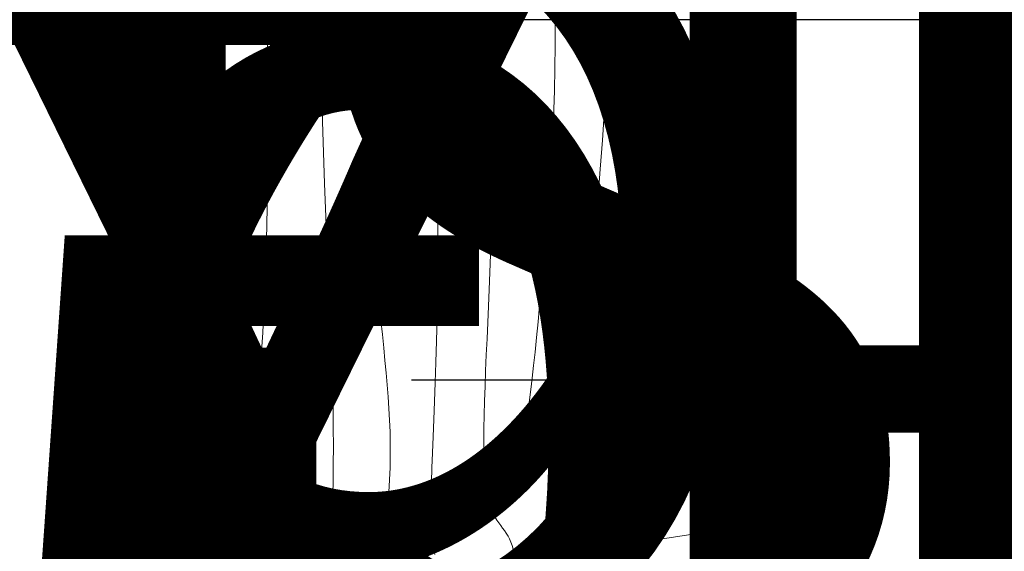
# Model space of a CAD drawing. Units: inches. Extents: x -307 to 2141, y -58 to 895.
# Tile 14 of 28: x 666 to 749, y 436 to 481. Entities that reach past the tile are written whole.
import ezdxf

# ---------------------------------------------------------------- set-up
doc = ezdxf.new("R2010")
doc.units = ezdxf.units.IN
doc.header["$MEASUREMENT"] = 0
doc.layers.add('A-ANNO-DIMS', color=2, linetype='Continuous', lineweight=18)
doc.layers.add('A-FURN', color=8, linetype='Continuous', lineweight=18)
doc.styles.get("Standard").update_dxf_attribs({"font": 'arial.ttf'})
doc.dimstyles.get("Standard").update_dxf_attribs({"dimtxt": 72, "dimasz": 48, "dimexe": 0.18, "dimexo": 0.0625, "dimgap": 0.09, "dimtad": 0, "dimtih": 1, "dimtoh": 1, "dimdec": 0, "dimrnd": 48, "dimzin": 0, "dimdsep": 46, "dimlunit": 3, "dimtxsty": 'Standard', "dimcen": 0.09, "dimadec": 0, "dimazin": 0, "dimtfac": 1, "dimtdec": 0, "dimtofl": 0, "dimtmove": 0, "dimatfit": 3, "dimfxl": 1, "dimtolj": 1, "dimtzin": 0, "dimarcsym": 0})

# ---------------------------------------------------------------- blocks, each defined once
blk = doc.blocks.new('Dining Set - 36 x 72 in.')
for p, q in [((-22, 27.5), (-6, 27.5)), ((-5.8437, 26.49966), (-6, 27.5)), ((6, 27.5), (5.8438, 26.50042)), ((6, 27.5), (22, 27.5)), ((22.1563, 26.49966), (22, 27.5)), ((-22.2304, 26), (-5.7608, 26)), ((-5.8416, 26.5), (-22.1534, 26.5)), ((-4.5152, 17.99762), (-5.7655, 25.99926)), ((5.7657, 26.00059), (4.5153, 17.99762)), ((5.7696, 26), (22.2392, 26)), ((22.1584, 26.5), (5.8466, 26.5)), ((23.4848, 17.99762), (22.2345, 25.99926)), ((36, 18), (-36, 18)), ((-36, -18), (36, -18)), ((-4.5152, -17.99762), (-5.7655, -25.99928)), ((5.7657, -26.0006), (4.5153, -17.99762)), ((23.4848, -17.99762), (22.2345, -25.99928)), ((-22.2304, -26), (-5.7608, -26)), ((-5.8416, -26.5), (-22.1534, -26.5)), ((-5.8437, -26.49967), (-6, -27.5)), ((5.7696, -26), (22.2392, -26)), ((6, -27.5), (5.8438, -26.50044)), ((22.1584, -26.5), (5.8466, -26.5)), ((22.1563, -26.49967), (22, -27.5)), ((-22, -27.5), (-6, -27.5)), ((6, -27.5), (22, -27.5))]:
    blk.add_line(p, q)
for points in [[(-22.8538, 14.81543), (-19.276, 14.6875), (-16.0362, 14.53613), (-13.0957, 14.36718), (-10.4159, 14.18652), (-7.9583, 14), (-5.6904, 13.81315), (-3.6035, 13.63021), (-1.6954, 13.45508), (0.0365, 13.29166), (1.5945, 13.14388), (2.9811, 13.01562), (4.1988, 12.9108), (5.25, 12.83333), (6.1393, 12.78613), (6.8802, 12.76823), (7.4883, 12.77767), (7.9792, 12.8125), (8.3685, 12.87077), (8.6719, 12.95052), (8.9049, 13.0498), (9.0833, 13.16666), (9.2205, 13.29899), (9.3216, 13.44401), (9.3895, 13.59879), (9.4271, 13.76041), (9.4373, 13.92594), (9.4232, 14.09245), (9.3875, 14.257), (9.3333, 14.41666), (9.2638, 14.56917), (9.1836, 14.71484), (9.0975, 14.85465), (9.0104, 14.98958), (8.9272, 15.1206), (8.8529, 15.2487), (8.7922, 15.37483), (8.75, 15.5), (8.7305, 15.62467), (8.7344, 15.74739), (8.7617, 15.86621), (8.8125, 15.97916), (8.8867, 16.08431), (8.9844, 16.17968), (9.1055, 16.26334), (9.25, 16.33333), (9.4189, 16.38802), (9.6172, 16.42708), (9.8506, 16.45052), (10.125, 16.45833), (10.4463, 16.45052), (10.8203, 16.42708), (11.2529, 16.38802), (11.75, 16.33333), (12.3184, 16.26318), (12.9694, 16.17838), (13.7151, 16.07991), (14.5677, 15.96875), (15.5395, 15.84586), (16.6426, 15.71224), (17.8893, 15.56884), (19.2917, 15.41666), (20.859, 15.25667), (22.5879, 15.08984), (24.4721, 14.91715)], [(-23.1725, 10.20442), (-18.4241, 10.19775), (-14.5677, 10.13541), (-11.4399, 10.03011), (-8.877, 9.89453), (-6.7154, 9.74137), (-4.7917, 9.58333), (-2.9698, 9.43082), (-1.2246, 9.28515), (0.4415, 9.14534), (2.026, 9.01041), (3.5266, 8.87939), (4.9408, 8.7513), (6.266, 8.62516), (7.5, 8.5), (8.6411, 8.37549), (9.6914, 8.2539), (10.6538, 8.13818), (11.5312, 8.03125), (12.3267, 7.93603), (13.043, 7.85547), (13.6831, 7.79248), (14.25, 7.75), (14.7471, 7.7303), (15.1797, 7.73307), (15.5537, 7.75732), (15.875, 7.80208), (16.1494, 7.86637), (16.3828, 7.94922), (16.5811, 8.04964), (16.75, 8.16666), (16.8944, 8.29915), (17.0143, 8.44531), (17.1089, 8.60319), (17.1771, 8.77083), (17.218, 8.94629), (17.2305, 9.1276), (17.2137, 9.31282), (17.1667, 9.5), (17.0895, 9.6875), (16.987, 9.875), (16.8649, 10.0625), (16.7292, 10.25), (16.5856, 10.4375), (16.4401, 10.625), (16.2985, 10.8125), (16.1667, 11), (16.05, 11.18733), (15.9518, 11.3737), (15.8752, 11.5581), (15.8229, 11.73958), (15.798, 11.91715), (15.8034, 12.08984), (15.842, 12.25667), (15.9167, 12.41666), (16.0295, 12.56836), (16.1784, 12.70833), (16.3605, 12.83268), (16.5729, 12.9375), (16.8127, 13.01888), (17.0768, 13.07291), (17.3625, 13.0957), (17.6667, 13.08333), (17.9894, 13.03312), (18.3418, 12.94726), (18.7382, 12.82918), (19.1927, 12.68229), (19.7195, 12.51001), (20.3327, 12.31575), (21.0465, 12.10294), (21.875, 11.875), (22.8357, 11.63354), (23.959, 11.37304), (25.2786, 11.08618)], [(-21.9946, 5.11767), (-18.4271, 5.05208), (-15.3009, 5.00602), (-12.5508, 4.97265), (-10.1112, 4.94515), (-7.9167, 4.91666), (-5.909, 4.88167), (-4.0586, 4.83984), (-2.3429, 4.79215), (-0.7396, 4.73958), (0.7739, 4.6831), (2.22, 4.6237), (3.6213, 4.56233), (5, 4.5), (6.373, 4.43782), (7.7344, 4.3776), (9.0723, 4.32129), (10.375, 4.27083), (11.6309, 4.22819), (12.8281, 4.19531), (13.9551, 4.17415), (15, 4.16666), (15.954, 4.17448), (16.819, 4.19791), (17.6001, 4.23698), (18.3021, 4.29166), (18.9299, 4.36198), (19.4883, 4.44791), (19.9823, 4.54948), (20.4167, 4.66666), (20.7969, 4.79899), (21.1302, 4.94401), (21.4245, 5.09879), (21.6875, 5.26041), (21.9271, 5.42594), (22.1511, 5.59245), (22.3672, 5.757), (22.5834, 5.91666), (22.8065, 6.06868), (23.0404, 6.21093), (23.2879, 6.34147), (23.5521, 6.45833), (23.8358, 6.55957), (24.142, 6.64323), (24.4735, 6.70735)], [(-21.6519, -0.16284), (-17.6563, 0.00521), (-14.0005, 0.12833), (-10.6523, 0.21289), (-7.5796, 0.26522), (-4.75, 0.29166), (-2.134, 0.29793), (0.2878, 0.28711), (2.5317, 0.26163), (4.6146, 0.22396), (6.5529, 0.17651), (8.3633, 0.12174), (10.0623, 0.06209), (11.6667, 0), (13.1899, -0.06201), (14.6341, -0.1211), (15.9982, -0.17432), (17.2813, -0.21875), (18.4823, -0.25147), (19.6003, -0.26953), (20.6343, -0.27002), (21.5834, -0.25), (22.4481, -0.20768), (23.2357, -0.14584), (23.9549, -0.06836), (24.6146, 0.02083)], [(-27.1843, -6.31267), (-20.084, -6.1263), (-14.469, -5.9419), (-10.1094, -5.76042), (-6.7752, -5.58285), (-4.2363, -5.41016), (-2.2629, -5.24333), (-0.625, -5.08334), (0.8708, -4.93099), (2.2715, -4.78646), (3.5872, -4.64974), (4.8281, -4.52084), (6.0046, -4.39974), (7.127, -4.28646), (8.2053, -4.18099), (9.25, -4.08334), (10.2705, -3.99382), (11.2734, -3.91407), (12.2647, -3.84603), (13.25, -3.79167), (14.2354, -3.75293), (15.2266, -3.73177), (16.2295, -3.73015), (17.25, -3.75), (18.2912, -3.79248), (19.3451, -3.85547), (20.4009, -3.93604), (21.4479, -4.03125), (22.4754, -4.13819), (23.4727, -4.25391), (24.4289, -4.37549)], [(-26.4022, -9.81299), (-18.4675, -9.62891), (-11.9839, -9.45069), (-6.7396, -9.28125), (-2.5226, -9.12354), (0.8789, -8.98047), (3.6769, -8.85498), (6.0833, -8.75), (8.2767, -8.66765), (10.3021, -8.60677), (12.1712, -8.56543), (13.8958, -8.54167), (15.4876, -8.53353), (16.9583, -8.53907), (18.3197, -8.55632), (19.5834, -8.58334), (20.7616, -8.61841), (21.8685, -8.66081), (22.9188, -8.71004), (23.9271, -8.76563), (24.9081, -8.82707)], [(-20.7312, -14.12647), (-17.0781, -14.07292), (-13.97, -14.04671), (-11.3027, -14.04297), (-8.9724, -14.05681), (-6.875, -14.08334), (-4.9224, -14.11833), (-3.0905, -14.16016), (-1.3709, -14.20785), (0.2448, -14.26042), (1.7647, -14.3169), (3.1973, -14.3763), (4.5507, -14.43767), (5.8333, -14.5), (7.0554, -14.5621), (8.235, -14.62175), (9.3922, -14.67652), (10.5469, -14.72396), (11.7192, -14.76164), (12.929, -14.78711), (14.1965, -14.79794), (15.5417, -14.79167), (16.9933, -14.76424), (18.6152, -14.70508), (20.4804, -14.60197), (22.6615, -14.44271), (25.2312, -14.21509)]]:
    blk.add_lwpolyline(points)
blk = doc.blocks.new('*D26')
at = {"layer": 'A-ANNO-DIMS', "color": 0, "lineweight": -2, "transparency": 16777216}
for p, q in [((565.336, 584.202), (565.336, 572.085)), ((645.336, 584.202), (645.336, 572.085)), ((517.336, 572.265), (469.336, 572.265)), ((693.336, 572.265), (741.336, 572.265))]:
    blk.add_line(p, q, dxfattribs=at)
at = {"layer": 'A-ANNO-DIMS', "color": 0, "transparency": 16777216}
for points in [[(517.336, 580.265), (517.336, 564.265), (565.336, 572.265)], [(693.336, 580.265), (693.336, 564.265), (645.336, 572.265)]]:
    blk.add_solid(points, dxfattribs=at)
at = {"layer": 'Defpoints', "color": 0, "transparency": 16777216}
for p in [(565.336, 584.265), (645.336, 584.265), (565.336, 572.265)]:
    blk.add_point(p, dxfattribs=at)
at = {"layer": 'A-ANNO-DIMS', "color": 0, "transparency": 16777216, "insert": (178.225, 572.265), "char_height": 72, "attachment_point": 5}
blk.add_mtext('\\A1;BED 80 TYP.', dxfattribs=at)
blk = doc.blocks.new('*D29')
at = {"layer": 'A-ANNO-DIMS', "color": 0, "lineweight": -2, "transparency": 16777216}
for p, q in [((747.421, 450.871), (699.421, 450.871)), ((795.421, 433.612), (795.421, 451.051)), ((882.028, 433.612), (882.028, 451.051)), ((930.028, 450.871), (978.028, 450.871))]:
    blk.add_line(p, q, dxfattribs=at)
at = {"layer": 'A-ANNO-DIMS', "color": 0, "transparency": 16777216}
for points in [[(747.421, 458.871), (747.421, 442.871), (795.421, 450.871)], [(930.028, 458.871), (930.028, 442.871), (882.028, 450.871)]]:
    blk.add_solid(points, dxfattribs=at)
at = {"layer": 'Defpoints', "color": 0, "transparency": 16777216}
for p in [(795.421, 450.871), (795.421, 433.55), (882.028, 433.55)]:
    blk.add_point(p, dxfattribs=at)
at = {"layer": 'A-ANNO-DIMS', "color": 0, "transparency": 16777216, "insert": (647.713, 450.871), "char_height": 72, "attachment_point": 5}
blk.add_mtext('\\A1;87', dxfattribs=at)
blk = doc.blocks.new('*D30')
at = {"layer": 'A-ANNO-DIMS', "color": 0, "lineweight": -2, "transparency": 16777216}
for p, q in [((570.736, 532.833), (570.736, 580.833)), ((570.736, 580.833), (618.736, 580.833)), ((565.398, 484.833), (570.916, 484.833)), ((565.398, 448.833), (570.916, 448.833)), ((570.736, 400.833), (570.736, 352.833))]:
    blk.add_line(p, q, dxfattribs=at)
at = {"layer": 'A-ANNO-DIMS', "color": 0, "transparency": 16777216}
for points in [[(562.736, 532.833), (578.736, 532.833), (570.736, 484.833)], [(562.736, 400.833), (578.736, 400.833), (570.736, 448.833)]]:
    blk.add_solid(points, dxfattribs=at)
at = {"layer": 'Defpoints', "color": 0, "transparency": 16777216}
for p in [(565.336, 484.833), (570.736, 484.833), (565.336, 448.833)]:
    blk.add_point(p, dxfattribs=at)
at = {"layer": 'A-ANNO-DIMS', "color": 0, "transparency": 16777216, "insert": (1030.174, 580.833), "char_height": 72, "attachment_point": 5}
blk.add_mtext('\\A1;WINDOW 36 TYP.', dxfattribs=at)
blk = doc.blocks.new('*D31')
at = {"layer": 'A-ANNO-DIMS', "color": 0, "lineweight": -2, "transparency": 16777216}
for p, q in [((556.336, 448.771), (556.336, 443.253)), ((565.336, 448.771), (565.336, 443.253)), ((508.336, 443.433), (460.336, 443.433)), ((613.336, 443.433), (661.336, 443.433))]:
    blk.add_line(p, q, dxfattribs=at)
at = {"layer": 'A-ANNO-DIMS', "color": 0, "transparency": 16777216}
for points in [[(508.336, 451.433), (508.336, 435.433), (556.336, 443.433)], [(613.336, 451.433), (613.336, 435.433), (565.336, 443.433)]]:
    blk.add_solid(points, dxfattribs=at)
at = {"layer": 'Defpoints', "color": 0, "transparency": 16777216}
for p in [(556.336, 448.833), (565.336, 448.833), (565.336, 443.433)]:
    blk.add_point(p, dxfattribs=at)
at = {"layer": 'A-ANNO-DIMS', "color": 0, "transparency": 16777216, "insert": (808.692, 443.433), "char_height": 72, "attachment_point": 5}
blk.add_mtext('\\A1;9 TYP.', dxfattribs=at)
blk = doc.blocks.new('*D35')
at = {"layer": 'A-ANNO-DIMS', "color": 0, "lineweight": -2, "transparency": 16777216}
for p, q in [((907.336, 443.029), (907.336, 453.949)), ((916.336, 443.029), (916.336, 453.949)), ((859.336, 453.769), (811.336, 453.769)), ((964.336, 453.769), (1012.336, 453.769))]:
    blk.add_line(p, q, dxfattribs=at)
at = {"layer": 'A-ANNO-DIMS', "color": 0, "transparency": 16777216}
for points in [[(859.336, 461.769), (859.336, 445.769), (907.336, 453.769)], [(964.336, 461.769), (964.336, 445.769), (916.336, 453.769)]]:
    blk.add_solid(points, dxfattribs=at)
at = {"layer": 'Defpoints', "color": 0, "transparency": 16777216}
for p in [(907.336, 453.769), (907.336, 442.967), (916.336, 442.967)]:
    blk.add_point(p, dxfattribs=at)
at = {"layer": 'A-ANNO-DIMS', "color": 0, "transparency": 16777216, "insert": (663.98, 453.769), "char_height": 72, "attachment_point": 5}
blk.add_mtext('\\A1;9 TYP.', dxfattribs=at)
blk = doc.blocks.new('*D36')
at = {"layer": 'A-ANNO-DIMS', "color": 0, "lineweight": -2, "transparency": 16777216}
for p, q in [((871.707, 562.404), (871.761, 610.404)), ((876.548, 514.399), (871.474, 514.405)), ((876.511, 481.353), (871.437, 481.358)), ((871.563, 433.358), (871.509, 385.358)), ((871.509, 385.358), (823.509, 385.358))]:
    blk.add_line(p, q, dxfattribs=at)
at = {"layer": 'A-ANNO-DIMS', "color": 0, "transparency": 16777216}
for points in [[(863.707, 562.413), (879.707, 562.395), (871.654, 514.404)], [(863.563, 433.367), (879.563, 433.349), (871.617, 481.358)]]:
    blk.add_solid(points, dxfattribs=at)
at = {"layer": 'Defpoints', "color": 0, "transparency": 16777216}
for p in [(876.611, 514.399), (871.617, 481.358), (876.574, 481.353)]:
    blk.add_point(p, dxfattribs=at)
at = {"layer": 'A-ANNO-DIMS', "color": 0, "transparency": 16777216, "insert": (548.95, 385.358), "char_height": 72, "attachment_point": 5}
blk.add_mtext('\\A1;WC 33 TYP.', dxfattribs=at)
blk = doc.blocks.new('*D37')
at = {"layer": 'A-ANNO-DIMS', "color": 0, "lineweight": -2, "transparency": 16777216}
for p, q in [((828.616, 519.409), (780.616, 519.463)), ((876.611, 514.461), (876.616, 519.536)), ((897.611, 514.438), (897.616, 519.512)), ((945.616, 519.279), (993.616, 519.225))]:
    blk.add_line(p, q, dxfattribs=at)
at = {"layer": 'A-ANNO-DIMS', "color": 0, "transparency": 16777216}
for points in [[(828.625, 527.409), (828.607, 511.409), (876.616, 519.356)], [(945.625, 527.279), (945.607, 511.279), (897.616, 519.332)]]:
    blk.add_solid(points, dxfattribs=at)
at = {"layer": 'Defpoints', "color": 0, "transparency": 16777216}
for p in [(876.616, 519.356), (876.611, 514.399), (897.611, 514.375)]:
    blk.add_point(p, dxfattribs=at)
at = {"layer": 'A-ANNO-DIMS', "color": 0, "transparency": 16777216, "insert": (604.676, 519.463), "char_height": 72, "attachment_point": 5}
blk.add_mtext('\\A1;21 TYP.', dxfattribs=at)
blk = doc.blocks.new('*D42')
at = {"layer": 'A-ANNO-DIMS', "color": 0, "lineweight": -2, "transparency": 16777216}
for p, q in [((880.259, 543.859), (928.248, 544.868)), ((832.299, 541.413), (832.265, 543.03)), ((822.302, 541.203), (822.268, 542.82)), ((774.282, 541.631), (726.293, 540.622))]:
    blk.add_line(p, q, dxfattribs=at)
at = {"layer": 'A-ANNO-DIMS', "color": 0, "transparency": 16777216}
for points in [[(880.09, 551.857), (880.427, 535.861), (832.269, 542.85)], [(774.114, 549.629), (774.45, 533.633), (822.271, 542.64)]]:
    blk.add_solid(points, dxfattribs=at)
at = {"layer": 'Defpoints', "color": 0, "transparency": 16777216}
for p in [(832.269, 542.85), (832.301, 541.35), (822.303, 541.14)]:
    blk.add_point(p, dxfattribs=at)
at = {"layer": 'A-ANNO-DIMS', "color": 0, "transparency": 16777216, "insert": (1192.886, 544.868), "char_height": 72, "attachment_point": 5}
blk.add_mtext('\\A1;FAUCET 10', dxfattribs=at)
blk = doc.blocks.new('*D43')
at = {"layer": 'A-ANNO-DIMS', "color": 0, "lineweight": -2, "transparency": 16777216}
for p, q in [((818.785, 637.088), (770.785, 637.088)), ((819.794, 589.098), (818.785, 637.088)), ((822.24, 541.139), (820.623, 541.105)), ((822.377, 534.64), (820.76, 534.606)), ((821.949, 486.621), (822.958, 438.631))]:
    blk.add_line(p, q, dxfattribs=at)
at = {"layer": 'A-ANNO-DIMS', "color": 0, "transparency": 16777216}
for points in [[(827.792, 589.266), (811.796, 588.93), (820.803, 541.109)], [(829.947, 486.789), (813.951, 486.453), (820.94, 534.61)]]:
    blk.add_solid(points, dxfattribs=at)
at = {"layer": 'Defpoints', "color": 0, "transparency": 16777216}
for p in [(820.803, 541.109), (822.303, 541.14), (822.44, 534.642)]:
    blk.add_point(p, dxfattribs=at)
at = {"layer": 'A-ANNO-DIMS', "color": 0, "transparency": 16777216, "insert": (747.391, 637.088), "char_height": 72, "attachment_point": 5}
blk.add_mtext('\\A1;7', dxfattribs=at)
blk = doc.blocks.new('*D44')
at = {"layer": 'A-ANNO-DIMS', "color": 0, "lineweight": -2, "transparency": 16777216}
for p, q in [((815.327, 520.707), (815.406, 516.907)), ((839.872, 521.223), (839.952, 517.424)), ((887.938, 518.613), (935.927, 519.622)), ((767.413, 516.078), (719.424, 515.069))]:
    blk.add_line(p, q, dxfattribs=at)
at = {"layer": 'A-ANNO-DIMS', "color": 0, "transparency": 16777216}
for points in [[(887.769, 526.611), (888.106, 510.614), (839.948, 517.604)], [(767.245, 524.076), (767.581, 508.08), (815.403, 517.087)]]:
    blk.add_solid(points, dxfattribs=at)
at = {"layer": 'Defpoints', "color": 0, "transparency": 16777216}
for p in [(815.325, 520.769), (839.871, 521.285), (839.948, 517.604)]:
    blk.add_point(p, dxfattribs=at)
at = {"layer": 'A-ANNO-DIMS', "color": 0, "transparency": 16777216, "insert": (1151.157, 519.622), "char_height": 72, "attachment_point": 5}
blk.add_mtext('\\A1;BASIN 25', dxfattribs=at)
blk = doc.blocks.new('*D45')
at = {"layer": 'A-ANNO-DIMS', "color": 0, "lineweight": -2, "transparency": 16777216}
for p, q in [((841.111, 637.474), (793.111, 637.474)), ((842.12, 589.484), (841.111, 637.474)), ((839.51, 541.419), (843.309, 541.499)), ((839.933, 521.287), (843.732, 521.367)), ((844.562, 473.373), (845.571, 425.384))]:
    blk.add_line(p, q, dxfattribs=at)
at = {"layer": 'A-ANNO-DIMS', "color": 0, "transparency": 16777216}
for points in [[(850.118, 589.652), (834.122, 589.316), (843.129, 541.495)], [(852.56, 473.542), (836.563, 473.205), (843.553, 521.363)]]:
    blk.add_solid(points, dxfattribs=at)
at = {"layer": 'Defpoints', "color": 0, "transparency": 16777216}
for p in [(839.447, 541.417), (843.129, 541.495), (839.871, 521.285)]:
    blk.add_point(p, dxfattribs=at)
at = {"layer": 'A-ANNO-DIMS', "color": 0, "transparency": 16777216, "insert": (740.961, 637.474), "char_height": 72, "attachment_point": 5}
blk.add_mtext('\\A1;20', dxfattribs=at)
blk = doc.blocks.new('*D46')
at = {"layer": 'A-ANNO-DIMS', "color": 0, "lineweight": -2, "transparency": 16777216}
for p, q in [((801.413, 645.783), (801.413, 642.516)), ((822.413, 645.783), (822.413, 642.516)), ((753.413, 642.696), (705.413, 642.696)), ((870.413, 642.696), (918.413, 642.696))]:
    blk.add_line(p, q, dxfattribs=at)
at = {"layer": 'A-ANNO-DIMS', "color": 0, "transparency": 16777216}
for points in [[(753.413, 650.696), (753.413, 634.696), (801.413, 642.696)], [(870.413, 650.696), (870.413, 634.696), (822.413, 642.696)]]:
    blk.add_solid(points, dxfattribs=at)
at = {"layer": 'Defpoints', "color": 0, "transparency": 16777216}
for p in [(801.413, 645.846), (822.413, 645.846), (822.413, 642.696)]:
    blk.add_point(p, dxfattribs=at)
at = {"layer": 'A-ANNO-DIMS', "color": 0, "transparency": 16777216, "insert": (1282.702, 642.696), "char_height": 72, "attachment_point": 5}
blk.add_mtext('\\A1;DESK CHAIR 21', dxfattribs=at)
blk = doc.blocks.new('*D51')
at = {"layer": 'A-ANNO-DIMS', "color": 0, "lineweight": -2, "transparency": 16777216}
for p, q in [((562.796, 379.109), (562.796, 427.109)), ((562.796, 427.109), (610.796, 427.109)), ((565.273, 331.109), (562.616, 331.109)), ((565.273, 315.867), (562.616, 315.867)), ((562.796, 267.867), (562.796, 219.867))]:
    blk.add_line(p, q, dxfattribs=at)
at = {"layer": 'A-ANNO-DIMS', "color": 0, "transparency": 16777216}
for points in [[(554.796, 379.109), (570.796, 379.109), (562.796, 331.109)], [(554.796, 267.867), (570.796, 267.867), (562.796, 315.867)]]:
    blk.add_solid(points, dxfattribs=at)
at = {"layer": 'Defpoints', "color": 0, "transparency": 16777216}
for p in [(562.796, 331.109), (565.336, 331.109), (565.336, 315.867)]:
    blk.add_point(p, dxfattribs=at)
at = {"layer": 'A-ANNO-DIMS', "color": 0, "transparency": 16777216, "insert": (659.336, 427.109), "char_height": 72, "attachment_point": 5}
blk.add_mtext('\\A1;15', dxfattribs=at)
blk = doc.blocks.new('*D52')
at = {"layer": 'A-ANNO-DIMS', "color": 0, "lineweight": -2, "transparency": 16777216}
for p, q in [((660.208, 554.249), (660.208, 602.249)), ((673.796, 506.249), (660.028, 506.249)), ((673.796, 415.249), (660.028, 415.249)), ((660.208, 367.249), (660.208, 319.249))]:
    blk.add_line(p, q, dxfattribs=at)
at = {"layer": 'A-ANNO-DIMS', "color": 0, "transparency": 16777216}
for points in [[(652.208, 554.249), (668.208, 554.249), (660.208, 506.249)], [(652.208, 367.249), (668.208, 367.249), (660.208, 415.249)]]:
    blk.add_solid(points, dxfattribs=at)
at = {"layer": 'Defpoints', "color": 0, "transparency": 16777216}
for p in [(673.858, 506.249), (660.208, 415.249), (673.858, 415.249)]:
    blk.add_point(p, dxfattribs=at)
at = {"layer": 'A-ANNO-DIMS', "color": 0, "transparency": 16777216, "insert": (660.208, 460.749), "char_height": 72, "attachment_point": 5}
blk.add_mtext('\\A1;DINING SET 91', dxfattribs=at)
blk = doc.blocks.new('*D53')
at = {"layer": 'A-ANNO-DIMS', "color": 0, "lineweight": -2, "transparency": 16777216}
for p, q in [((673.858, 415.186), (673.858, 401.419)), ((728.858, 415.186), (728.858, 401.419)), ((625.858, 401.599), (577.858, 401.599)), ((776.858, 401.599), (824.858, 401.599))]:
    blk.add_line(p, q, dxfattribs=at)
at = {"layer": 'A-ANNO-DIMS', "color": 0, "transparency": 16777216}
for points in [[(625.858, 409.599), (625.858, 393.599), (673.858, 401.599)], [(776.858, 409.599), (776.858, 393.599), (728.858, 401.599)]]:
    blk.add_solid(points, dxfattribs=at)
at = {"layer": 'Defpoints', "color": 0, "transparency": 16777216}
for p in [(673.858, 415.249), (728.858, 415.249), (728.858, 401.599)]:
    blk.add_point(p, dxfattribs=at)
at = {"layer": 'A-ANNO-DIMS', "color": 0, "transparency": 16777216, "insert": (876.787, 401.599), "char_height": 72, "attachment_point": 5}
blk.add_mtext('\\A1;55', dxfattribs=at)
blk = doc.blocks.new('*D54')
at = {"layer": 'A-ANNO-DIMS', "color": 0, "lineweight": -2, "transparency": 16777216}
for p, q in [((605.336, 412.349), (605.336, 460.349)), ((605.336, 460.349), (653.336, 460.349)), ((596.398, 364.349), (605.516, 364.349)), ((596.398, 304.349), (605.516, 304.349)), ((605.336, 256.349), (605.336, 208.349))]:
    blk.add_line(p, q, dxfattribs=at)
at = {"layer": 'A-ANNO-DIMS', "color": 0, "transparency": 16777216}
for points in [[(597.336, 412.349), (613.336, 412.349), (605.336, 364.349)], [(597.336, 256.349), (613.336, 256.349), (605.336, 304.349)]]:
    blk.add_solid(points, dxfattribs=at)
at = {"layer": 'Defpoints', "color": 0, "transparency": 16777216}
for p in [(596.336, 364.349), (605.336, 364.349), (596.336, 304.349)]:
    blk.add_point(p, dxfattribs=at)
at = {"layer": 'A-ANNO-DIMS', "color": 0, "transparency": 16777216, "insert": (854.004, 460.349), "char_height": 72, "attachment_point": 5}
blk.add_mtext('\\A1;DESK 60', dxfattribs=at)
blk = doc.blocks.new('*D60')
at = {"layer": 'A-ANNO-DIMS', "color": 0, "lineweight": -2, "transparency": 16777216}
for p, q in [((659.857, 294.946), (659.857, 342.946)), ((659.857, 342.946), (707.857, 342.946)), ((663.339, 246.946), (659.677, 246.946)), ((663.339, 223.315), (659.677, 223.315)), ((659.857, 175.315), (659.857, 127.315))]:
    blk.add_line(p, q, dxfattribs=at)
at = {"layer": 'A-ANNO-DIMS', "color": 0, "transparency": 16777216}
for points in [[(651.857, 294.946), (667.857, 294.946), (659.857, 246.946)], [(651.857, 175.315), (667.857, 175.315), (659.857, 223.315)]]:
    blk.add_solid(points, dxfattribs=at)
at = {"layer": 'Defpoints', "color": 0, "transparency": 16777216}
for p in [(659.857, 246.946), (663.402, 246.946), (663.402, 223.315)]:
    blk.add_point(p, dxfattribs=at)
at = {"layer": 'A-ANNO-DIMS', "color": 0, "transparency": 16777216, "insert": (933.573, 342.946), "char_height": 72, "attachment_point": 5}
blk.add_mtext('\\A1;TABLE 24', dxfattribs=at)
blk = doc.blocks.new('*D63')
at = {"layer": 'A-ANNO-DIMS', "color": 0, "lineweight": -2, "transparency": 16777216}
for p, q in [((916.398, 691.341), (947.72, 691.341)), ((947.54, 643.341), (947.54, 416.192)), ((947.54, 115.341), (947.54, 342.49)), ((704.684, 67.341), (947.72, 67.341))]:
    blk.add_line(p, q, dxfattribs=at)
at = {"layer": 'A-ANNO-DIMS', "color": 0, "transparency": 16777216}
for points in [[(939.54, 643.341), (955.54, 643.341), (947.54, 691.341)], [(939.54, 115.341), (955.54, 115.341), (947.54, 67.341)]]:
    blk.add_solid(points, dxfattribs=at)
at = {"layer": 'Defpoints', "color": 0, "transparency": 16777216}
for p in [(916.336, 691.341), (704.621, 67.341), (947.54, 67.341)]:
    blk.add_point(p, dxfattribs=at)
at = {"layer": 'A-ANNO-DIMS', "color": 0, "transparency": 16777216, "insert": (947.54, 379.341), "char_height": 72, "attachment_point": 5}
blk.add_mtext('\\A1;624', dxfattribs=at)
blk = doc.blocks.new('*D68')
at = {"layer": 'A-ANNO-DIMS', "color": 0, "lineweight": -2, "transparency": 16777216}
for p, q in [((525.132, 586.341), (525.132, 634.341)), ((525.132, 634.341), (573.132, 634.341)), ((565.273, 538.341), (524.952, 538.341)), ((556.273, 484.833), (524.952, 484.833)), ((525.132, 436.833), (525.132, 388.833))]:
    blk.add_line(p, q, dxfattribs=at)
at = {"layer": 'A-ANNO-DIMS', "color": 0, "transparency": 16777216}
for points in [[(517.132, 586.341), (533.132, 586.341), (525.132, 538.341)], [(517.132, 436.833), (533.132, 436.833), (525.132, 484.833)]]:
    blk.add_solid(points, dxfattribs=at)
at = {"layer": 'Defpoints', "color": 0, "transparency": 16777216}
for p in [(525.132, 538.341), (565.336, 538.341), (556.336, 484.833)]:
    blk.add_point(p, dxfattribs=at)
at = {"layer": 'A-ANNO-DIMS', "color": 0, "transparency": 16777216, "insert": (687.754, 634.341), "char_height": 72, "attachment_point": 5}
blk.add_mtext('\\A1;53.51', dxfattribs=at)
blk = doc.blocks.new('*D82')
at = {"layer": 'A-ANNO-DIMS', "color": 0, "lineweight": -2, "transparency": 16777216}
for p, q in [((525.132, 565.341), (525.132, 613.341)), ((525.132, 613.341), (573.132, 613.341)), ((802.273, 517.341), (524.952, 517.341)), ((802.273, 481.341), (524.952, 481.341)), ((525.132, 433.341), (525.132, 385.341))]:
    blk.add_line(p, q, dxfattribs=at)
at = {"layer": 'A-ANNO-DIMS', "color": 0, "transparency": 16777216}
for points in [[(517.132, 565.341), (533.132, 565.341), (525.132, 517.341)], [(517.132, 433.341), (533.132, 433.341), (525.132, 481.341)]]:
    blk.add_solid(points, dxfattribs=at)
at = {"layer": 'Defpoints', "color": 0, "transparency": 16777216}
for p in [(525.132, 517.341), (802.336, 517.341), (802.336, 481.341)]:
    blk.add_point(p, dxfattribs=at)
at = {"layer": 'A-ANNO-DIMS', "color": 0, "transparency": 16777216, "insert": (624.742, 613.341), "char_height": 72, "attachment_point": 5}
blk.add_mtext('\\A1;36', dxfattribs=at)
blk = doc.blocks.new('*D83')
at = {"layer": 'A-ANNO-DIMS', "color": 0, "lineweight": -2, "transparency": 16777216}
for p, q in [((947.54, 538.903), (947.54, 586.903)), ((916.398, 490.903), (947.72, 490.903)), ((907.398, 481.341), (947.72, 481.341)), ((947.54, 433.341), (947.54, 385.341)), ((947.54, 385.341), (899.54, 385.341))]:
    blk.add_line(p, q, dxfattribs=at)
at = {"layer": 'A-ANNO-DIMS', "color": 0, "transparency": 16777216}
for points in [[(939.54, 538.903), (955.54, 538.903), (947.54, 490.903)], [(939.54, 433.341), (955.54, 433.341), (947.54, 481.341)]]:
    blk.add_solid(points, dxfattribs=at)
at = {"layer": 'Defpoints', "color": 0, "transparency": 16777216}
for p in [(916.336, 490.903), (907.336, 481.341), (947.54, 481.341)]:
    blk.add_point(p, dxfattribs=at)
at = {"layer": 'A-ANNO-DIMS', "color": 0, "transparency": 16777216, "insert": (777.968, 385.341), "char_height": 72, "attachment_point": 5}
blk.add_mtext('\\A1;9.563', dxfattribs=at)
blk = doc.blocks.new('*D88')
at = {"layer": 'A-ANNO-DIMS', "color": 0, "lineweight": -2, "transparency": 16777216}
for p, q in [((517.33584, 722.544828), (469.33584, 722.544828)), ((565.33584, 295.403328), (565.33584, 722.724828)), ((754.33584, 271.403328), (754.33584, 722.724828)), ((802.33584, 722.544828), (850.33584, 722.544828))]:
    blk.add_line(p, q, dxfattribs=at)
at = {"layer": 'A-ANNO-DIMS', "color": 0, "transparency": 16777216}
for points in [[(517.33584, 730.544828), (517.33584, 714.544828), (565.33584, 722.544828)], [(802.33584, 730.544828), (802.33584, 714.544828), (754.33584, 722.544828)]]:
    blk.add_solid(points, dxfattribs=at)
at = {"layer": 'Defpoints', "color": 0, "transparency": 16777216}
for p in [(754.33584, 722.544828), (565.33584, 295.340828), (754.33584, 271.340828)]:
    blk.add_point(p, dxfattribs=at)
at = {"layer": 'A-ANNO-DIMS', "color": 0, "transparency": 16777216, "insert": (659.83584, 722.544828), "char_height": 72, "attachment_point": 5}
blk.add_mtext('\\A1;189', dxfattribs=at)
blk = doc.blocks.new('*D95')
at = {"layer": 'A-ANNO-DIMS', "color": 0, "lineweight": -2, "transparency": 16777216}
for p, q in [((947.54, 577.341), (947.54, 625.341)), ((947.54, 625.341), (995.54, 625.341)), ((629.898, 529.341), (947.72, 529.341)), ((629.898, 502.663), (947.72, 502.663)), ((947.54, 454.663), (947.54, 406.663))]:
    blk.add_line(p, q, dxfattribs=at)
at = {"layer": 'A-ANNO-DIMS', "color": 0, "transparency": 16777216}
for points in [[(939.54, 577.341), (955.54, 577.341), (947.54, 529.341)], [(939.54, 454.663), (955.54, 454.663), (947.54, 502.663)]]:
    blk.add_solid(points, dxfattribs=at)
at = {"layer": 'Defpoints', "color": 0, "transparency": 16777216}
for p in [(629.836, 529.341), (947.54, 529.341), (629.836, 502.663)]:
    blk.add_point(p, dxfattribs=at)
at = {"layer": 'A-ANNO-DIMS', "color": 0, "transparency": 16777216, "insert": (1117.799, 625.341), "char_height": 72, "attachment_point": 5}
blk.add_mtext('\\A1;26.68', dxfattribs=at)
blk = doc.blocks.new('*D97')
at = {"layer": 'A-ANNO-DIMS', "color": 0, "lineweight": -2, "transparency": 16777216}
for p, q in [((947.54, 637.341), (947.54, 685.341)), ((947.54, 685.341), (995.54, 685.341)), ((685.398, 589.341), (947.72, 589.341)), ((685.398, 538.341), (947.72, 538.341)), ((947.54, 490.341), (947.54, 442.341))]:
    blk.add_line(p, q, dxfattribs=at)
at = {"layer": 'A-ANNO-DIMS', "color": 0, "transparency": 16777216}
for points in [[(939.54, 637.341), (955.54, 637.341), (947.54, 589.341)], [(939.54, 490.341), (955.54, 490.341), (947.54, 538.341)]]:
    blk.add_solid(points, dxfattribs=at)
at = {"layer": 'Defpoints', "color": 0, "transparency": 16777216}
for p in [(685.336, 589.341), (947.54, 589.341), (685.336, 538.341)]:
    blk.add_point(p, dxfattribs=at)
at = {"layer": 'A-ANNO-DIMS', "color": 0, "transparency": 16777216, "insert": (1040.249, 685.341), "char_height": 72, "attachment_point": 5}
blk.add_mtext('\\A1;51', dxfattribs=at)
blk = doc.blocks.new('*D98')
at = {"layer": 'A-ANNO-DIMS', "color": 0, "lineweight": -2, "transparency": 16777216}
for p, q in [((525.132, 637.341), (525.132, 685.341)), ((525.132, 685.341), (573.132, 685.341)), ((787.273, 589.341), (524.952, 589.341)), ((787.273, 550.341), (524.952, 550.341)), ((525.132, 502.341), (525.132, 454.341))]:
    blk.add_line(p, q, dxfattribs=at)
at = {"layer": 'A-ANNO-DIMS', "color": 0, "transparency": 16777216}
for points in [[(517.132, 637.341), (533.132, 637.341), (525.132, 589.341)], [(517.132, 502.341), (533.132, 502.341), (525.132, 550.341)]]:
    blk.add_solid(points, dxfattribs=at)
at = {"layer": 'Defpoints', "color": 0, "transparency": 16777216}
for p in [(525.132, 589.341), (787.336, 589.341), (787.336, 550.341)]:
    blk.add_point(p, dxfattribs=at)
at = {"layer": 'A-ANNO-DIMS', "color": 0, "transparency": 16777216, "insert": (624.84, 685.341), "char_height": 72, "attachment_point": 5}
blk.add_mtext('\\A1;39', dxfattribs=at)
blk = doc.blocks.new('*D99')
at = {"layer": 'A-ANNO-DIMS', "color": 0, "lineweight": -2, "transparency": 16777216}
for p, q in [((763.336, 481.278), (763.336, 35.957)), ((802.336, 481.278), (802.336, 35.957)), ((715.336, 36.137), (667.336, 36.137)), ((850.336, 36.137), (898.336, 36.137))]:
    blk.add_line(p, q, dxfattribs=at)
at = {"layer": 'A-ANNO-DIMS', "color": 0, "transparency": 16777216}
for points in [[(715.336, 44.137), (715.336, 28.137), (763.336, 36.137)], [(850.336, 44.137), (850.336, 28.137), (802.336, 36.137)]]:
    blk.add_solid(points, dxfattribs=at)
at = {"layer": 'Defpoints', "color": 0, "transparency": 16777216}
for p in [(763.336, 481.341), (802.336, 481.341), (802.336, 36.137)]:
    blk.add_point(p, dxfattribs=at)
at = {"layer": 'A-ANNO-DIMS', "color": 0, "transparency": 16777216, "insert": (950.044, 36.137), "char_height": 72, "attachment_point": 5}
blk.add_mtext('\\A1;39', dxfattribs=at)
blk = doc.blocks.new('*D107')
at = {"layer": 'A-ANNO-DIMS', "color": 0, "lineweight": -2, "transparency": 16777216}
for p, q in [((517.336, 722.545), (469.336, 722.545)), ((565.336, 409.403), (565.336, 722.725)), ((589.339, 409.403), (589.339, 722.725)), ((637.339, 722.545), (685.339, 722.545))]:
    blk.add_line(p, q, dxfattribs=at)
at = {"layer": 'A-ANNO-DIMS', "color": 0, "transparency": 16777216}
for points in [[(517.336, 730.545), (517.336, 714.545), (565.336, 722.545)], [(637.339, 730.545), (637.339, 714.545), (589.339, 722.545)]]:
    blk.add_solid(points, dxfattribs=at)
at = {"layer": 'Defpoints', "color": 0, "transparency": 16777216}
for p in [(589.339, 722.545), (565.336, 409.341), (589.339, 409.341)]:
    blk.add_point(p, dxfattribs=at)
at = {"layer": 'A-ANNO-DIMS', "color": 0, "transparency": 16777216, "insert": (835.495, 722.545), "char_height": 72, "attachment_point": 5}
blk.add_mtext('\\A1;24.003', dxfattribs=at)
blk = doc.blocks.new('*D108')
at = {"layer": 'A-ANNO-DIMS', "color": 0, "lineweight": -2, "transparency": 16777216}
for p, q in [((947.54, 550.663), (947.54, 598.663)), ((589.402, 502.663), (947.72, 502.663)), ((589.402, 409.341), (947.72, 409.341)), ((947.54, 361.341), (947.54, 313.341))]:
    blk.add_line(p, q, dxfattribs=at)
at = {"layer": 'A-ANNO-DIMS', "color": 0, "transparency": 16777216}
for points in [[(939.54, 550.663), (955.54, 550.663), (947.54, 502.663)], [(939.54, 361.341), (955.54, 361.341), (947.54, 409.341)]]:
    blk.add_solid(points, dxfattribs=at)
at = {"layer": 'Defpoints', "color": 0, "transparency": 16777216}
for p in [(589.339, 502.663), (947.54, 502.663), (589.339, 409.341)]:
    blk.add_point(p, dxfattribs=at)
at = {"layer": 'A-ANNO-DIMS', "color": 0, "transparency": 16777216, "insert": (947.54, 456.002), "char_height": 72, "attachment_point": 5}
blk.add_mtext('\\A1;93.32', dxfattribs=at)
blk = doc.blocks.new('*D109')
at = {"layer": 'A-ANNO-DIMS', "color": 0, "lineweight": -2, "transparency": 16777216}
for p, q in [((723.132, 355.341), (723.132, 403.341)), ((723.132, 403.341), (771.132, 403.341)), ((754.273, 307.341), (722.952, 307.341)), ((754.273, 271.341), (722.952, 271.341)), ((723.132, 223.341), (723.132, 175.341))]:
    blk.add_line(p, q, dxfattribs=at)
at = {"layer": 'A-ANNO-DIMS', "color": 0, "transparency": 16777216}
for points in [[(715.132, 355.341), (731.132, 355.341), (723.132, 307.341)], [(715.132, 223.341), (731.132, 223.341), (723.132, 271.341)]]:
    blk.add_solid(points, dxfattribs=at)
at = {"layer": 'Defpoints', "color": 0, "transparency": 16777216}
for p in [(723.132, 307.341), (754.336, 307.341), (754.336, 271.341)]:
    blk.add_point(p, dxfattribs=at)
at = {"layer": 'A-ANNO-DIMS', "color": 0, "transparency": 16777216, "insert": (822.742, 403.341), "char_height": 72, "attachment_point": 5}
blk.add_mtext('\\A1;36', dxfattribs=at)

msp = doc.modelspace()

# ---------------------------------------------------------------- block references
at = {"layer": 'A-FURN', "rotation": 270}
msp.add_blockref('Dining Set - 36 x 72 in.', (701.3583, 460.7485), dxfattribs=at)

# ---------------------------------------------------------------- dimensions: what is measured, and where the dimension line sits
at = {"layer": 'A-ANNO-DIMS'}
for base, p1, p2, text, picture, middle in [((822.4132, 642.696), (801.4132, 645.846), (822.4132, 645.846), 'DESK CHAIR <>', '*D46', (1282.7024, 642.696)), ((565.3358, 443.4333), (556.3358, 448.8333), (565.3358, 448.8333), '<> TYP.', '*D31', (808.6919, 443.4333))]:
    dim = msp.add_linear_dim(base=base, p1=p1, p2=p2, text=text, dimstyle='Standard', override={"dimdec": 0, "dimlfac": 1, "dimrnd": 0, "dimzin": 0, "dimdsep": 46, "dimlunit": 2}, dxfattribs=at)
    dim.commit()
    dim.dimension.update_dxf_attribs({"geometry": picture, "text_midpoint": middle})
for base, p1, p2, override, picture, middle in [((754.3358, 722.5448), (565.3358, 295.3408), (754.3358, 271.3408), {"dimdec": 0, "dimlfac": 1, "dimrnd": 0, "dimzin": 0, "dimdsep": 46, "dimlunit": 2}, '*D88', (659.8358, 722.5448)), ((589.339, 722.5448), (565.3358, 409.3408), (589.339, 409.3408), {"dimdec": 3, "dimlfac": 1, "dimrnd": 0, "dimzin": 0, "dimdsep": 46, "dimlunit": 2}, '*D107', (835.4945, 722.5448)), ((802.3358, 36.1368), (763.3358, 481.3408), (802.3358, 481.3408), {"dimdec": 0, "dimlfac": 1, "dimrnd": 0, "dimzin": 0, "dimdsep": 46, "dimlunit": 2}, '*D99', (950.0438, 36.1368)), ((728.8583, 401.5985), (673.8583, 415.2485), (728.8583, 415.2485), {"dimdec": 0, "dimlfac": 1, "dimrnd": 0, "dimzin": 0, "dimdsep": 46, "dimlunit": 2}, '*D53', (876.7874, 401.5985))]:
    dim = msp.add_linear_dim(base=base, p1=p1, p2=p2, dimstyle='Standard', override=override, dxfattribs=at)
    dim.commit()
    dim.dimension.update_dxf_attribs({"geometry": picture, "text_midpoint": middle})
for base, p1, p2, angle, text, picture, middle in [((570.7358, 484.8333), (565.3358, 448.8333), (565.3358, 484.8333), 90, 'WINDOW <> TYP.', '*D30', (1030.1737, 580.8333)), ((565.3358, 572.2648), (645.3359, 584.2648), (565.3358, 584.2648), 180, 'BED <> TYP.', '*D26', (178.2254, 572.2648)), ((832.2692, 542.8502), (822.3029, 541.1403), (832.3007, 541.3505), 1.204628, 'FAUCET <>', '*D42', (1192.8864, 544.8684)), ((660.2083, 415.2485), (673.8583, 506.2485), (673.8583, 415.2485), 270, 'DINING SET <>', '*D52', (660.2083, 460.7485)), ((839.9481, 517.6035), (815.3253, 520.7692), (839.8707, 521.2853), 1.204628, 'BASIN <>', '*D44', (1151.1574, 519.6217)), ((876.6162, 519.3557), (897.6106, 514.3753), (876.6106, 514.3988), 179.935892, '<> TYP.', '*D37', (604.6763, 519.4631)), ((871.6167, 481.3581), (876.6106, 514.3988), (876.5736, 481.3526), 269.935892, 'WC <> TYP.', '*D36', (548.95, 385.3582)), ((605.3358, 364.3488), (596.3358, 304.3488), (596.3358, 364.3488), 90, 'DESK <>', '*D54', (854.0043, 460.3488)), ((907.3358, 453.7692), (916.3358, 442.9669), (907.3358, 442.9669), 180, '<> TYP.', '*D35', (663.9798, 453.7692)), ((659.8571, 246.9465), (663.4018, 223.3153), (663.4018, 246.9465), 90, 'TABLE <>', '*D60', (933.5733, 342.9465))]:
    dim = msp.add_linear_dim(base=base, p1=p1, p2=p2, angle=angle, text=text, dimstyle='Standard', override={"dimdec": 0, "dimlfac": 1, "dimrnd": 0, "dimzin": 0, "dimdsep": 46, "dimlunit": 2}, dxfattribs=at)
    dim.commit()
    dim.dimension.update_dxf_attribs({"geometry": picture, "text_midpoint": middle})
for base, p1, p2, angle, override, picture, middle in [((525.1318, 589.3408), (787.3358, 550.3408), (787.3358, 589.3408), 90, {"dimdec": 0, "dimlfac": 1, "dimrnd": 0, "dimzin": 0, "dimdsep": 46, "dimlunit": 2}, '*D98', (624.8398, 685.3408)), ((947.5398, 589.3408), (685.3358, 538.3408), (685.3358, 589.3408), 90, {"dimdec": 0, "dimlfac": 1, "dimrnd": 0, "dimzin": 0, "dimdsep": 46, "dimlunit": 2}, '*D97', (1040.2492, 685.3408)), ((947.5398, 67.3408), (916.3358, 691.3408), (704.6211, 67.3408), 90, {"dimdec": 0, "dimlfac": 1, "dimrnd": 0, "dimzin": 0, "dimdsep": 46, "dimlunit": 2}, '*D63', (947.5398, 379.3408)), ((843.1292, 541.4949), (839.8707, 521.2853), (839.4474, 541.4175), 91.204628, {"dimdec": 0, "dimlfac": 1, "dimrnd": 0, "dimzin": 0, "dimdsep": 46, "dimlunit": 2}, '*D45', (740.961, 637.4737)), ((820.8033, 541.1087), (822.4396, 534.6416), (822.3029, 541.1403), 91.204628, {"dimdec": 0, "dimlfac": 1, "dimrnd": 0, "dimzin": 0, "dimdsep": 46, "dimlunit": 2}, '*D43', (747.3908, 637.0875)), ((525.1318, 538.3408), (556.3358, 484.8333), (565.3358, 538.3408), 90, {"dimdec": 2, "dimlfac": 1, "dimrnd": 0, "dimzin": 0, "dimdsep": 46, "dimlunit": 2}, '*D68', (687.7539, 634.3408)), ((947.5398, 529.3408), (629.8358, 502.6632), (629.8358, 529.3408), 90, {"dimdec": 2, "dimlfac": 1, "dimrnd": 0, "dimzin": 0, "dimdsep": 46, "dimlunit": 2}, '*D95', (1117.799, 625.3408)), ((525.1318, 517.3408), (802.3358, 481.3408), (802.3358, 517.3408), 90, {"dimdec": 0, "dimlfac": 1, "dimrnd": 0, "dimzin": 0, "dimdsep": 46, "dimlunit": 2}, '*D82', (624.7416, 613.3408)), ((947.5398, 502.6632), (589.339, 409.3408), (589.339, 502.6632), 90, {"dimdec": 2, "dimlfac": 1, "dimrnd": 0, "dimzin": 0, "dimdsep": 46, "dimlunit": 2}, '*D108', (947.5398, 456.002)), ((947.5398, 481.3408), (916.3358, 490.9034), (907.3358, 481.3408), 90, {"dimdec": 3, "dimlfac": 1, "dimrnd": 0, "dimzin": 0, "dimdsep": 46, "dimlunit": 2}, '*D83', (777.9683, 385.3408)), ((795.4208, 450.8711), (882.0282, 433.5496), (795.4208, 433.5496), 180, {"dimdec": 0, "dimlfac": 1, "dimrnd": 0, "dimzin": 0, "dimdsep": 46, "dimlunit": 2}, '*D29', (647.7128, 450.8711)), ((562.7955, 331.1086), (565.3358, 315.8666), (565.3358, 331.1086), 90, {"dimdec": 0, "dimlfac": 1, "dimrnd": 0, "dimzin": 0, "dimdsep": 46, "dimlunit": 2}, '*D51', (659.3357, 427.1086)), ((723.1318, 307.3408), (754.3358, 271.3408), (754.3358, 307.3408), 90, {"dimdec": 0, "dimlfac": 1, "dimrnd": 0, "dimzin": 0, "dimdsep": 46, "dimlunit": 2}, '*D109', (822.7416, 403.3408))]:
    dim = msp.add_linear_dim(base=base, p1=p1, p2=p2, angle=angle, dimstyle='Standard', override=override, dxfattribs=at)
    dim.commit()
    dim.dimension.update_dxf_attribs({"geometry": picture, "text_midpoint": middle})

doc.saveas('drawing.dxf')
